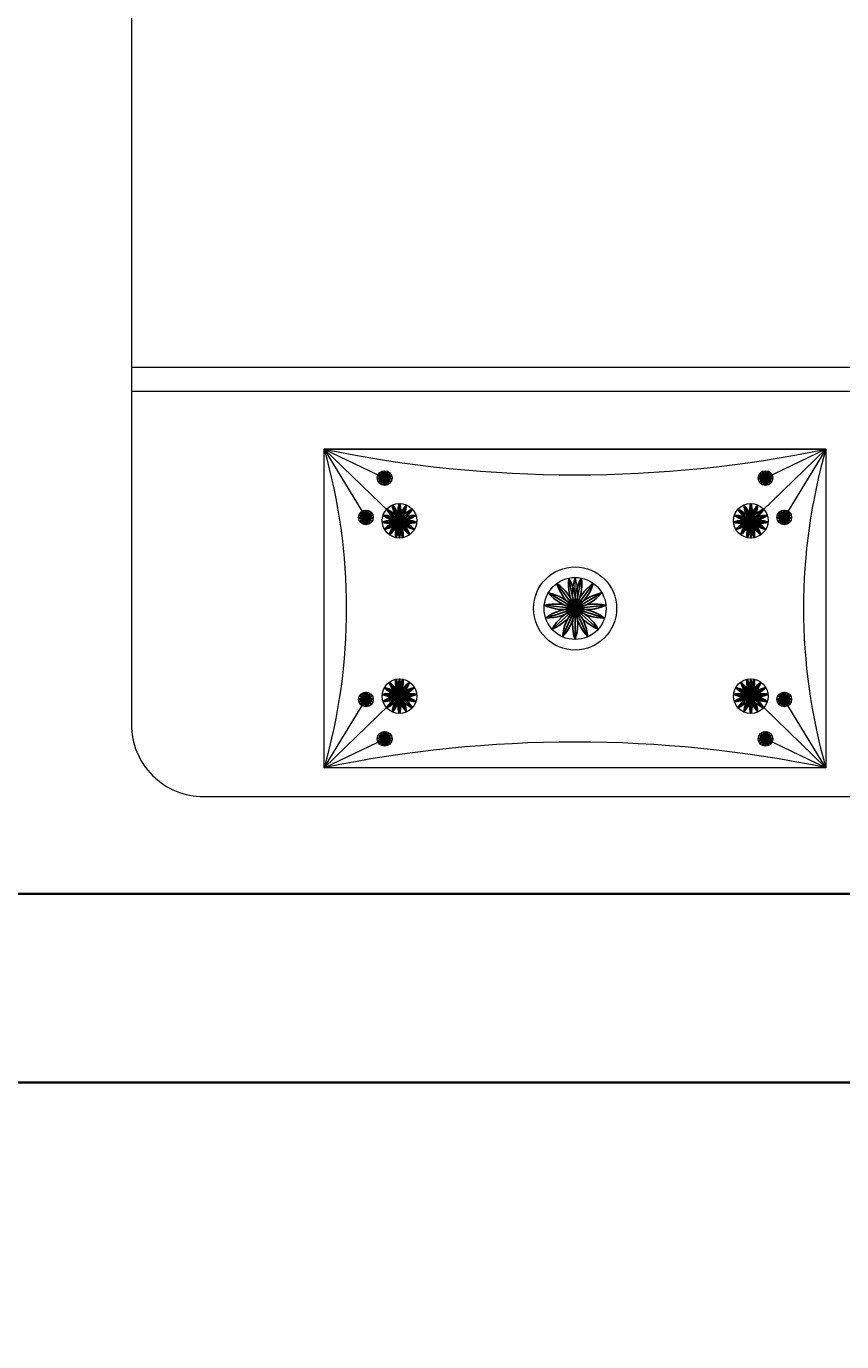
# Model space of a CAD drawing. Units: inches. Extents: x -61 to 1599, y -1316 to 257.
# Tile 186 of 204: x 1088 to 1126, y -454 to -391. Entities that reach past the tile are written whole.
import ezdxf

# ---------------------------------------------------------------- set-up
doc = ezdxf.new("R2010")
doc.units = ezdxf.units.IN
doc.header["$MEASUREMENT"] = 0
for name, color, linetype, lineweight in [('A-ANNO-DIMS', 2, 'Continuous', 18), ('FURNITURE', 83, 'Continuous', 18), ('WALLS', 4, 'Continuous', 35)]:
    doc.layers.add(name, color=color, linetype=linetype, lineweight=lineweight)
doc.layers.add('LT', color=8, linetype='Continuous')
doc.styles.get("Standard").update_dxf_attribs({"font": 'arial.ttf'})
doc.dimstyles.get("Standard").update_dxf_attribs({"dimtxt": 0.18, "dimasz": 0.18, "dimexe": 0.18, "dimexo": 0.0625, "dimgap": 0.09, "dimtad": 0, "dimtih": 1, "dimtoh": 1, "dimdec": 0, "dimzin": 0, "dimdsep": 46, "dimlunit": 3, "dimtxsty": 'Standard', "dimcen": 0.09, "dimadec": 0, "dimazin": 0, "dimtfac": 1, "dimtdec": 0, "dimtofl": 0, "dimtmove": 0, "dimatfit": 3, "dimfxl": 1, "dimtolj": 1, "dimtzin": 0, "dimarcsym": 0})

# ---------------------------------------------------------------- blocks, each defined once
blk = doc.blocks.new('*U15')
at = {"layer": 'LT'}
blk.add_line((0, 0.175), (0, -0.175), dxfattribs=at)
for centre, start, end in [((0.509, 0), 160.9983, 199.0017), ((-0.509, 0), 340.9983, 19.0017)]:
    blk.add_arc(centre, 0.539, start, end, dxfattribs=at)
blk = doc.blocks.new('*U16')
at = {"layer": 'LT', "transparency": 16777216}
for p, rotation in [((-66.649, -18.828), 96), ((-66.642, -18.755), 72), ((-66.627, -18.897), 120), ((-66.605, -18.692), 48.00000000000001), ((-66.578, -18.951), 144), ((-66.546, -18.649), 24), ((-66.512, -18.981), 168.0000000000001), ((-66.439, -18.981), 192), ((-66.404, -18.649), 336.0000000000001), ((-66.372, -18.951), 216), ((-66.345, -18.692), 312), ((-66.323, -18.897), 240), ((-66.308, -18.755), 288.0000000000001), ((-66.301, -18.828), 264)]:
    blk.add_blockref('*U15', p, dxfattribs=dict(at, rotation=rotation))
blk.add_blockref('*U15', (-66.475, -18.634), dxfattribs=at)
blk = doc.blocks.new('*U45')
at = {"layer": 'LT'}
blk.add_line((0, 0.175), (0, -0.175), dxfattribs=at)
for centre, start, end in [((0.509, 0), 160.9983, 199.0017), ((-0.509, 0), 340.9983, 19.0017)]:
    blk.add_arc(centre, 0.539, start, end, dxfattribs=at)
blk = doc.blocks.new('*U46')
at = {"layer": 'LT', "transparency": 16777216}
for p, rotation in [((-66.649, -18.828), 96), ((-66.642, -18.755), 72), ((-66.627, -18.897), 120), ((-66.605, -18.692), 48.00000000000001), ((-66.578, -18.951), 144), ((-66.546, -18.649), 24), ((-66.512, -18.981), 168.0000000000001), ((-66.439, -18.981), 192), ((-66.404, -18.649), 336.0000000000001), ((-66.372, -18.951), 216), ((-66.345, -18.692), 312), ((-66.323, -18.897), 240), ((-66.308, -18.755), 288.0000000000001), ((-66.301, -18.828), 264)]:
    blk.add_blockref('*U45', p, dxfattribs=dict(at, rotation=rotation))
blk.add_blockref('*U45', (-66.475, -18.634), dxfattribs=at)
blk = doc.blocks.new('*U9')
at = {"layer": 'LT'}
blk.add_line((0, 0.175), (0, -0.175), dxfattribs=at)
for centre, start, end in [((0.509, 0), 160.9983, 199.0017), ((-0.509, 0), 340.9983, 19.0017)]:
    blk.add_arc(centre, 0.539, start, end, dxfattribs=at)
blk = doc.blocks.new('*U10')
at = {"layer": 'LT', "transparency": 16777216}
for p, rotation in [((-66.649, -18.828), 96), ((-66.642, -18.755), 72), ((-66.627, -18.897), 120), ((-66.605, -18.692), 48.00000000000001), ((-66.578, -18.951), 144), ((-66.546, -18.649), 24), ((-66.512, -18.981), 168.0000000000001), ((-66.439, -18.981), 192), ((-66.404, -18.649), 336.0000000000001), ((-66.372, -18.951), 216), ((-66.345, -18.692), 312), ((-66.323, -18.897), 240), ((-66.308, -18.755), 288.0000000000001), ((-66.301, -18.828), 264)]:
    blk.add_blockref('*U9', p, dxfattribs=dict(at, rotation=rotation))
blk.add_blockref('*U9', (-66.475, -18.634), dxfattribs=at)
blk = doc.blocks.new('*U39')
at = {"layer": 'LT'}
blk.add_line((0, 0.175), (0, -0.175), dxfattribs=at)
for centre, start, end in [((0.509, 0), 160.9983, 199.0017), ((-0.509, 0), 340.9983, 19.0017)]:
    blk.add_arc(centre, 0.539, start, end, dxfattribs=at)
blk = doc.blocks.new('*U40')
at = {"layer": 'LT', "transparency": 16777216}
for p, rotation in [((-66.649, -18.828), 96), ((-66.642, -18.755), 72), ((-66.627, -18.897), 120), ((-66.605, -18.692), 48.00000000000001), ((-66.578, -18.951), 144), ((-66.546, -18.649), 24), ((-66.512, -18.981), 168.0000000000001), ((-66.439, -18.981), 192), ((-66.404, -18.649), 336.0000000000001), ((-66.372, -18.951), 216), ((-66.345, -18.692), 312), ((-66.323, -18.897), 240), ((-66.308, -18.755), 288.0000000000001), ((-66.301, -18.828), 264)]:
    blk.add_blockref('*U39', p, dxfattribs=dict(at, rotation=rotation))
blk.add_blockref('*U39', (-66.475, -18.634), dxfattribs=at)
blk = doc.blocks.new('*U17')
at = {"layer": 'LT'}
blk.add_line((0, 0.412), (0, -0.412), dxfattribs=at)
for centre, start, end in [((1.198, 0), 160.9983, 199.0017), ((-1.198, 0), 340.9983, 19.0017)]:
    blk.add_arc(centre, 1.267, start, end, dxfattribs=at)
blk = doc.blocks.new('*U18')
at = {"layer": 'LT', "transparency": 16777216}
for p, rotation in [((-156.639, -43.959), 48.00000000000001), ((-156.501, -43.858), 24), ((-156.165, -43.858), 336.0000000000001), ((-156.027, -43.959), 312), ((-156.743, -44.278), 96), ((-156.725, -44.108), 72), ((-156.69, -44.441), 120), ((-156.575, -44.569), 144), ((-156.419, -44.639), 168), ((-156.247, -44.639), 192), ((-156.091, -44.569), 216), ((-155.976, -44.441), 240), ((-155.941, -44.108), 288.0000000000001), ((-155.923, -44.278), 264)]:
    blk.add_blockref('*U17', p, dxfattribs=dict(at, rotation=rotation))
blk.add_blockref('*U17', (-156.333, -43.823), dxfattribs=at)
blk = doc.blocks.new('*U33')
at = {"layer": 'LT'}
blk.add_line((0, 0.412), (0, -0.412), dxfattribs=at)
for centre, start, end in [((1.198, 0), 160.9983, 199.0017), ((-1.198, 0), 340.9983, 19.0017)]:
    blk.add_arc(centre, 1.267, start, end, dxfattribs=at)
blk = doc.blocks.new('*U34')
at = {"layer": 'LT', "transparency": 16777216}
for p, rotation in [((-156.639, -43.959), 48.00000000000001), ((-156.501, -43.858), 24), ((-156.165, -43.858), 336.0000000000001), ((-156.027, -43.959), 312), ((-156.743, -44.278), 96), ((-156.725, -44.108), 72), ((-156.69, -44.441), 120), ((-156.575, -44.569), 144), ((-156.419, -44.639), 168), ((-156.247, -44.639), 192), ((-156.091, -44.569), 216), ((-155.976, -44.441), 240), ((-155.941, -44.108), 288.0000000000001), ((-155.923, -44.278), 264)]:
    blk.add_blockref('*U33', p, dxfattribs=dict(at, rotation=rotation))
blk.add_blockref('*U33', (-156.333, -43.823), dxfattribs=at)
blk = doc.blocks.new('*U11')
at = {"layer": 'LT'}
blk.add_line((0, 0.739), (0, -0.739), dxfattribs=at)
for centre, start, end in [((2.147, 0), 160.9983, 199.0017), ((-2.147, 0), 340.9983, 19.0017)]:
    blk.add_arc(centre, 2.27, start, end, dxfattribs=at)
blk = doc.blocks.new('*U12')
at = {"layer": 'LT', "transparency": 16777216}
for p, rotation in [((-280.791, -78.801), 48.00000000000001), ((-280.542, -78.621), 23.99999999999999), ((-279.941, -78.621), 336.0000000000001), ((-279.692, -78.801), 312), ((-280.945, -79.067), 72), ((-279.539, -79.067), 288.0000000000001), ((-280.977, -79.373), 96), ((-280.882, -79.665), 120), ((-280.676, -79.894), 144), ((-280.395, -80.019), 168), ((-280.088, -80.019), 191.9999999999999), ((-279.807, -79.894), 216), ((-279.602, -79.665), 240), ((-279.507, -79.373), 264)]:
    blk.add_blockref('*U11', p, dxfattribs=dict(at, rotation=rotation))
blk.add_blockref('*U11', (-280.242, -78.557), dxfattribs=at)
blk = doc.blocks.new('*U28')
at = {"layer": 'LT'}
blk.add_line((0, 0.412), (0, -0.412), dxfattribs=at)
for centre, start, end in [((1.198, 0), 160.9983, 199.0017), ((-1.198, 0), 340.9983, 19.0017)]:
    blk.add_arc(centre, 1.267, start, end, dxfattribs=at)
blk = doc.blocks.new('*U44')
at = {"layer": 'LT', "transparency": 16777216}
for p, rotation in [((-156.639, -43.959), 48.00000000000001), ((-156.501, -43.858), 24), ((-156.165, -43.858), 336.0000000000001), ((-156.027, -43.959), 312), ((-156.743, -44.278), 96), ((-156.725, -44.108), 72), ((-156.69, -44.441), 120), ((-156.575, -44.569), 144), ((-156.419, -44.639), 168), ((-156.247, -44.639), 192), ((-156.091, -44.569), 216), ((-155.976, -44.441), 240), ((-155.941, -44.108), 288.0000000000001), ((-155.923, -44.278), 264)]:
    blk.add_blockref('*U28', p, dxfattribs=dict(at, rotation=rotation))
blk.add_blockref('*U28', (-156.333, -43.823), dxfattribs=at)
blk = doc.blocks.new('*U13')
at = {"layer": 'LT'}
blk.add_line((0, 0.412), (0, -0.412), dxfattribs=at)
for centre, start, end in [((1.198, 0), 160.9983, 199.0017), ((-1.198, 0), 340.9983, 19.0017)]:
    blk.add_arc(centre, 1.267, start, end, dxfattribs=at)
blk = doc.blocks.new('*U14')
at = {"layer": 'LT', "transparency": 16777216}
for p, rotation in [((-156.639, -43.959), 48.00000000000001), ((-156.501, -43.858), 24), ((-156.165, -43.858), 336.0000000000001), ((-156.027, -43.959), 312), ((-156.743, -44.278), 96), ((-156.725, -44.108), 72), ((-156.69, -44.441), 120), ((-156.575, -44.569), 144), ((-156.419, -44.639), 168), ((-156.247, -44.639), 192), ((-156.091, -44.569), 216), ((-155.976, -44.441), 240), ((-155.941, -44.108), 288.0000000000001), ((-155.923, -44.278), 264)]:
    blk.add_blockref('*U13', p, dxfattribs=dict(at, rotation=rotation))
blk.add_blockref('*U13', (-156.333, -43.823), dxfattribs=at)
blk = doc.blocks.new('*U19')
at = {"layer": 'LT'}
blk.add_line((0, 0.175), (0, -0.175), dxfattribs=at)
for centre, start, end in [((0.509, 0), 160.9983, 199.0017), ((-0.509, 0), 340.9983, 19.0017)]:
    blk.add_arc(centre, 0.539, start, end, dxfattribs=at)
blk = doc.blocks.new('*U6')
at = {"layer": 'LT', "transparency": 16777216}
for p, rotation in [((-66.649, -18.828), 96), ((-66.642, -18.755), 72), ((-66.627, -18.897), 120), ((-66.605, -18.692), 48.00000000000001), ((-66.578, -18.951), 144), ((-66.546, -18.649), 24), ((-66.512, -18.981), 168.0000000000001), ((-66.439, -18.981), 192), ((-66.404, -18.649), 336.0000000000001), ((-66.372, -18.951), 216), ((-66.345, -18.692), 312), ((-66.323, -18.897), 240), ((-66.308, -18.755), 288.0000000000001), ((-66.301, -18.828), 264)]:
    blk.add_blockref('*U19', p, dxfattribs=dict(at, rotation=rotation))
blk.add_blockref('*U19', (-66.475, -18.634), dxfattribs=at)
blk = doc.blocks.new('*U35')
at = {"layer": 'LT'}
blk.add_line((0, 0.175), (0, -0.175), dxfattribs=at)
for centre, start, end in [((0.509, 0), 160.9983, 199.0017), ((-0.509, 0), 340.9983, 19.0017)]:
    blk.add_arc(centre, 0.539, start, end, dxfattribs=at)
blk = doc.blocks.new('*U36')
at = {"layer": 'LT', "transparency": 16777216}
for p, rotation in [((-66.649, -18.828), 96), ((-66.642, -18.755), 72), ((-66.627, -18.897), 120), ((-66.605, -18.692), 48.00000000000001), ((-66.578, -18.951), 144), ((-66.546, -18.649), 24), ((-66.512, -18.981), 168.0000000000001), ((-66.439, -18.981), 192), ((-66.404, -18.649), 336.0000000000001), ((-66.372, -18.951), 216), ((-66.345, -18.692), 312), ((-66.323, -18.897), 240), ((-66.308, -18.755), 288.0000000000001), ((-66.301, -18.828), 264)]:
    blk.add_blockref('*U35', p, dxfattribs=dict(at, rotation=rotation))
blk.add_blockref('*U35', (-66.475, -18.634), dxfattribs=at)
blk = doc.blocks.new('*U7')
at = {"layer": 'LT'}
blk.add_line((0, 0.175), (0, -0.175), dxfattribs=at)
for centre, start, end in [((0.509, 0), 160.9983, 199.0017), ((-0.509, 0), 340.9983, 19.0017)]:
    blk.add_arc(centre, 0.539, start, end, dxfattribs=at)
blk = doc.blocks.new('*U8')
at = {"layer": 'LT', "transparency": 16777216}
for p, rotation in [((-66.649, -18.828), 96), ((-66.642, -18.755), 72), ((-66.627, -18.897), 120), ((-66.605, -18.692), 48.00000000000001), ((-66.578, -18.951), 144), ((-66.546, -18.649), 24), ((-66.512, -18.981), 168.0000000000001), ((-66.439, -18.981), 192), ((-66.404, -18.649), 336.0000000000001), ((-66.372, -18.951), 216), ((-66.345, -18.692), 312), ((-66.323, -18.897), 240), ((-66.308, -18.755), 288.0000000000001), ((-66.301, -18.828), 264)]:
    blk.add_blockref('*U7', p, dxfattribs=dict(at, rotation=rotation))
blk.add_blockref('*U7', (-66.475, -18.634), dxfattribs=at)
blk = doc.blocks.new('*U37')
at = {"layer": 'LT'}
blk.add_line((0, 0.175), (0, -0.175), dxfattribs=at)
for centre, start, end in [((0.509, 0), 160.9983, 199.0017), ((-0.509, 0), 340.9983, 19.0017)]:
    blk.add_arc(centre, 0.539, start, end, dxfattribs=at)
blk = doc.blocks.new('*U38')
at = {"layer": 'LT', "transparency": 16777216}
for p, rotation in [((-66.649, -18.828), 96), ((-66.642, -18.755), 72), ((-66.627, -18.897), 120), ((-66.605, -18.692), 48.00000000000001), ((-66.578, -18.951), 144), ((-66.546, -18.649), 24), ((-66.512, -18.981), 168.0000000000001), ((-66.439, -18.981), 192), ((-66.404, -18.649), 336.0000000000001), ((-66.372, -18.951), 216), ((-66.345, -18.692), 312), ((-66.323, -18.897), 240), ((-66.308, -18.755), 288.0000000000001), ((-66.301, -18.828), 264)]:
    blk.add_blockref('*U37', p, dxfattribs=dict(at, rotation=rotation))
blk.add_blockref('*U37', (-66.475, -18.634), dxfattribs=at)
blk = doc.blocks.new('BED-DOUBLE')
for p, q in [((1.272, 20.467), (70.263, 20.467)), ((1.272, 19.317), (70.263, 19.317)), ((10.471, 1.379), (10.471, 16.557)), ((34.388, 16.557), (10.471, 16.557)), ((10.471, 16.557), (13.35, 15.18)), ((10.471, 16.557), (14.039, 13.107)), ((10.471, 16.557), (12.454, 13.305)), ((34.388, 16.557), (30.82, 13.107)), ((34.388, 16.557), (31.508, 15.18)), ((34.388, 16.557), (32.405, 13.305)), ((13.35, 15.18), (13.35, 14.829)), ((31.508, 15.18), (31.508, 14.829)), ((12.454, 13.305), (12.454, 12.955)), ((32.405, 13.305), (32.405, 12.955)), ((14.052, 13.149), (14.052, 12.324)), ((30.806, 13.149), (30.806, 12.324)), ((22.429, 8.968), (22.429, 10.447)), ((14.052, 4.788), (14.052, 5.613)), ((30.806, 4.788), (30.806, 5.613)), ((10.471, 1.379), (14.039, 4.83)), ((10.471, 1.379), (12.454, 4.631)), ((12.454, 4.631), (12.454, 4.982)), ((34.388, 1.379), (30.82, 4.83)), ((32.405, 4.631), (32.405, 4.982)), ((34.388, 1.379), (32.405, 4.631)), ((10.471, 1.379), (13.35, 2.756)), ((13.35, 2.756), (13.35, 3.107)), ((31.508, 2.756), (31.508, 3.107)), ((34.388, 1.379), (31.508, 2.756)), ((34.388, 1.379), (34.388, 1.379))]:
    blk.add_line(p, q)
for points in [[(1.272, 88.537), (1.272, 3.449, 0.414214), (4.722, 0), (66.813, 0, 0.414214), (70.263, 3.449), (70.263, 88.537, 0.414214), (66.813, 91.987), (4.722, 91.987, 0.414214)], [(13.35, 15.18, 0.167358), (13.35, 14.829, 0.167358)], [(12.454, 13.305, 0.167358), (12.454, 12.955, 0.167358)], [(32.405, 12.955, 0.167358), (32.405, 13.305, 0.167358)], [(14.052, 13.149, 0.167358), (14.052, 12.324, 0.167358)], [(30.806, 12.324, 0.167358), (30.806, 13.149, 0.167358)], [(22.429, 8.968, 0.167358), (22.429, 10.447, 0.167358)], [(14.052, 5.613, 0.167358), (14.052, 4.788, 0.167358)], [(30.806, 4.788, 0.167358), (30.806, 5.613, 0.167358)], [(12.454, 4.982, 0.167358), (12.454, 4.631, 0.167358)], [(32.405, 4.631, 0.167358), (32.405, 4.982, 0.167358)], [(13.35, 3.107, 0.167358), (13.35, 2.756, 0.167358)], [(31.508, 2.756, 0.167358), (31.508, 3.107, 0.167358)]]:
    blk.add_lwpolyline(points, format="xyb", close=True)
blk.add_lwpolyline([(34.388, 16.557), (34.388, 1.379), (10.471, 1.379), (10.471, 16.557), (34.388, 16.557), (34.388, 1.379), (10.471, 1.379)])
for centre, radius in [((13.35, 15.18), 0.351), ((31.508, 15.18), 0.351), ((14.052, 13.149), 0.825), ((30.806, 13.149), 0.825), ((12.454, 13.305), 0.351), ((32.405, 13.305), 0.351), ((22.429, 8.968), 1.982), ((22.429, 8.968), 1.478), ((14.052, 4.788), 0.825), ((30.806, 4.788), 0.825), ((12.454, 4.631), 0.351), ((32.405, 4.631), 0.351), ((13.35, 2.756), 0.351), ((31.508, 2.756), 0.351)]:
    blk.add_circle(centre, radius)
for centre, radius, start, end in [((-16.003, 8.968), 27.54, 344.0046, 15.9954), ((22.429, 74.54), 59.203, 258.34678, 281.65322), ((60.861, 8.968), 27.54, 164.0046, 195.9954), ((32.017, 15.005), 0.539, 160.9983, 199.0017), ((30.999, 15.005), 0.539, 340.9983, 19.0017), ((22.429, -56.603), 59.203, 78.34678, 101.65322)]:
    blk.add_arc(centre, radius, start, end)
for name, p in [('*U40', (79.825, 33.99)), ('*U34', (170.385, 57.384)), ('*U46', (78.929, 32.115))]:
    blk.add_blockref(name, p)
at = {"extrusion": (0, 0, -1), "zscale": -1}
for name, p in [('*U36', (34.967, 33.99)), ('*U14', (125.527, 57.384)), ('*U38', (34.07, 32.115))]:
    blk.add_blockref(name, p, dxfattribs=at)
at = {"rotation": 180}
for name, p in [('*U12', (-257.812, -70.328)), ('*U44', (-125.527, -39.447)), ('*U8', (-34.07, -14.178)), ('*U6', (-34.967, -16.053))]:
    blk.add_blockref(name, p, dxfattribs=at)
at = {"extrusion": (0, 0, -1), "zscale": -1, "rotation": 180}
for name, p in [('*U18', (-170.385, -39.447)), ('*U16', (-78.929, -14.178)), ('*U10', (-79.825, -16.053))]:
    blk.add_blockref(name, p, dxfattribs=at)
blk = doc.blocks.new('*D698')
at = {"layer": 'A-ANNO-DIMS', "color": 0, "lineweight": -2, "transparency": 16777216}
for p, q in [((644.765, -167.169), (1598.483, -167.169)), ((1598.303, -167.349), (1598.303, -363.987)), ((1598.303, -560.989), (1598.303, -364.351)), ((644.765, -561.169), (1598.483, -561.169))]:
    blk.add_line(p, q, dxfattribs=at)
at = {"layer": 'A-ANNO-DIMS', "color": 0, "transparency": 16777216}
for points in [[(1598.273, -167.349), (1598.333, -167.349), (1598.303, -167.169)], [(1598.273, -560.989), (1598.333, -560.989), (1598.303, -561.169)]]:
    blk.add_solid(points, dxfattribs=at)
at = {"layer": 'DEFPOINTS', "color": 0, "transparency": 16777216}
for p in [(644.703, -167.169), (1598.303, -167.169), (644.703, -561.169)]:
    blk.add_point(p, dxfattribs=at)
at = {"layer": 'A-ANNO-DIMS', "color": 0, "transparency": 16777216, "insert": (1598.303, -364.169), "char_height": 0.18, "attachment_point": 5}
blk.add_mtext('\\A1;394', dxfattribs=at)

msp = doc.modelspace()

# ---------------------------------------------------------------- linework, layer by layer
at = {"layer": 'WALLS'}
for p, q in [((1065.7028, -432.3229), (1215.7028, -432.3229)), ((992.7028, -441.3229), (1215.7028, -441.3229))]:
    msp.add_line(p, q, dxfattribs=at)

# ---------------------------------------------------------------- block references
at = {"layer": 'FURNITURE'}
msp.add_blockref('BED-DOUBLE', (1091.2612, -427.6961), dxfattribs=at)

# ---------------------------------------------------------------- dimensions: what is measured, and where the dimension line sits
at = {"layer": 'A-ANNO-DIMS'}
dim = msp.add_linear_dim(base=(1598.3028, -167.169), p1=(644.7028, -561.169), p2=(644.7028, -167.169), angle=90, dimstyle='Standard', override={"dimdec": 0, "dimlfac": 1, "dimrnd": 0, "dimzin": 0, "dimdsep": 46, "dimlunit": 2}, dxfattribs=at)
dim.commit()
dim.dimension.update_dxf_attribs({"geometry": '*D698', "text_midpoint": (1598.3028, -364.169)})

doc.saveas('drawing.dxf')
